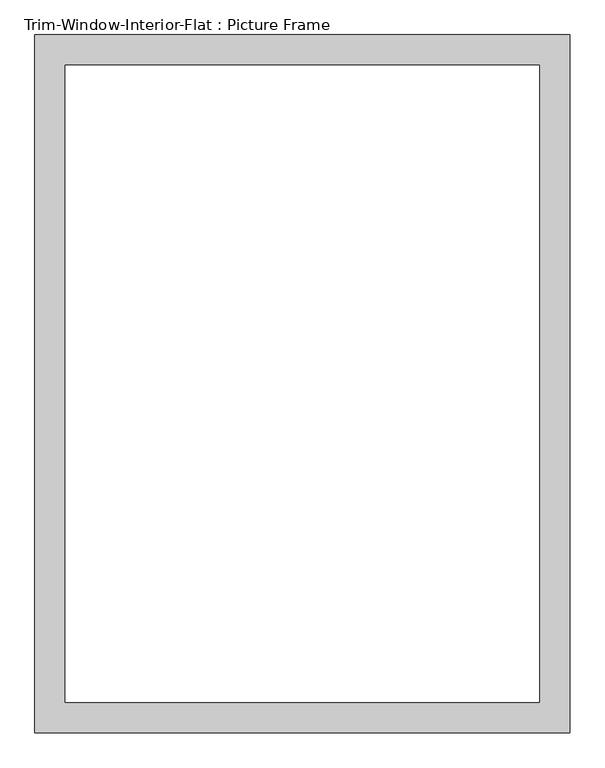
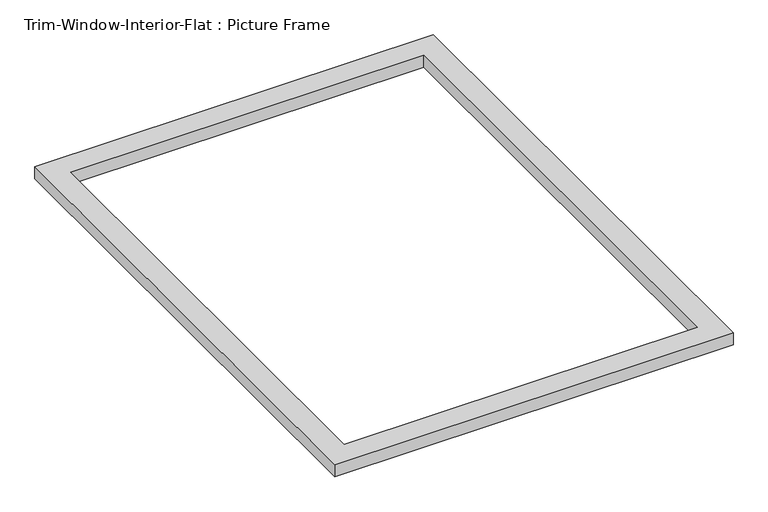
"""IFC4 building model written with IfcOpenShell, lengths in millimetres: proxy geometry, Trim-Window-Interior-Flat : Picture Frame."""

from ifc_helpers import new_model, si_unit, origin, origin_with_axes, place, context, project, spatial, polyline, outline, extrude, source, transform, mapped, element, save


def trim_window_interior_flat_picture_frame_39ff4276(model_context):
    return source(origin(), model_context, "Body", "SweptSolid", [
        extrude(outline(polyline([(501.65, 44.45), (501.65, -1263.65), (-501.65, -1263.65), (-501.65, 44.45), (501.65, 44.45)]), holes=[polyline([(444.5, -12.7), (-444.5, -12.7), (-444.5, -1206.5), (444.5, -1206.5), (444.5, -12.7)])]), origin_with_axes(), (0.0, 0.0, 1.0), 31.75),
    ])


if __name__ == "__main__":
    model = new_model("IFC4")
    model_context = context("Model", 3, world=origin())
    ifc_project = project(units=[si_unit("LENGTHUNIT", "METRE", prefix="MILLI")], contexts=[model_context])
    site = spatial("IfcSite", under=ifc_project)
    building = spatial("IfcBuilding", under=site)
    placement = place(None, origin())
    trim_window_interior_flat_picture_frame_shape = trim_window_interior_flat_picture_frame_39ff4276(model_context)
    element("IfcBuildingElementProxy", 1, Name="Trim-Window-Interior-Flat : Picture Frame", ObjectType="Trim-Window-Interior-Flat : Picture Frame", at=placement, inside=building, context=model_context, shape_type="MappedRepresentation", body=[
        mapped(trim_window_interior_flat_picture_frame_shape, transform((0.0, 0.0, 0.0), x_axis=(1.0, 0.0, 0.0), y_axis=(0.0, 1.0, 0.0), z_axis=(0.0, 0.0, 1.0))),
    ])
    save(model, "model.ifc")

# Revit data of these elements
# Type "Trim-Window-Interior-Flat : Picture Frame"
#   Trim Thickness_Picture Frame = 0' - 1 1/4"
#   Trim Width = 0' - 2 1/4"
#   Trim Thickness_with Sill = 0' - 0 3/4"
#   Sill Thickness = 0' - 1 1/4"
#   Opening Width [instance default] = 2' - 0"
#   Opening Height [instance default] = 3' - 0"
#   Default Elevation = 4' - 0"
#   Sill = no
#   Picture Frame = yes
#   Trim Material [instance default] = none
# Element 1 (IfcBuildingElementProxy, "Trim-Window-Interior-Flat : Picture Frame")
#   Opening Width = 3' - 0"
#   Opening Height = 4' - 0"
